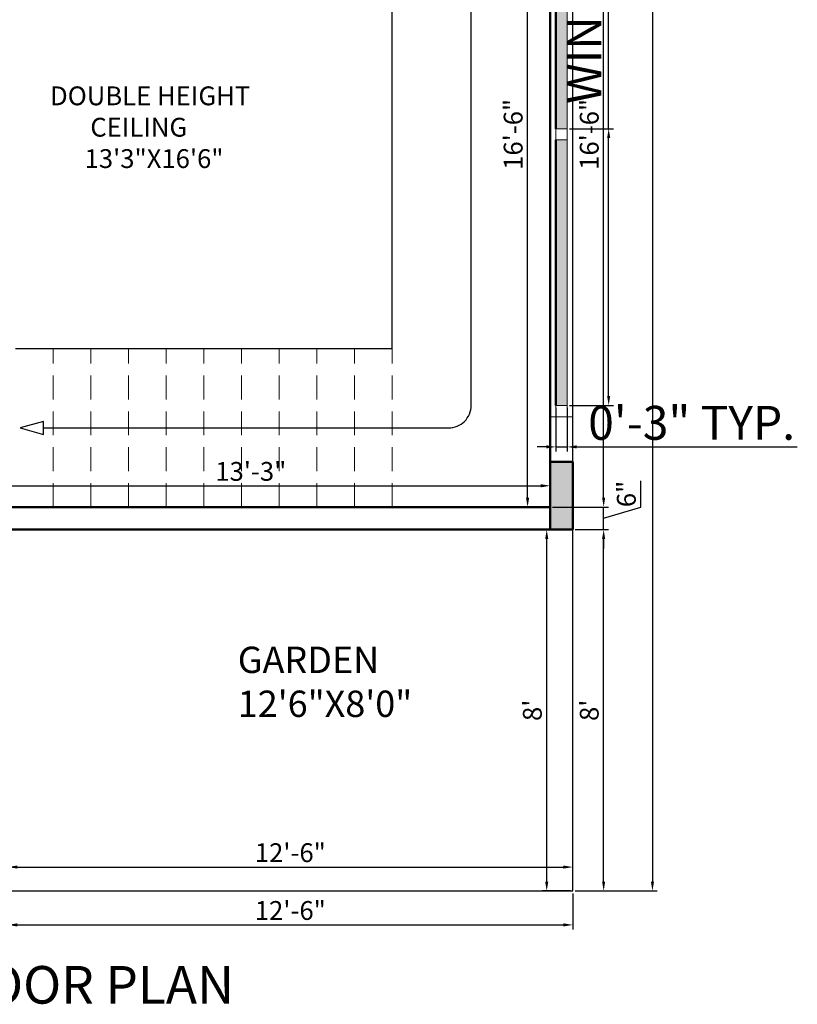
# Model space of a CAD drawing. Units: inches. Extents: x 3064 to 19385, y 846 to 15425.
# Tile 83 of 108: x 7295 to 7501, y 850 to 1112. Entities that reach past the tile are written whole.
import ezdxf

# ---------------------------------------------------------------- set-up
doc = ezdxf.new("R2010")
doc.units = ezdxf.units.IN
doc.linetypes.add('DASHED', pattern=[19.05, 12.7, -6.35])
for name, color, linetype, lineweight in [('A-ANNO-DIMS', 2, 'Continuous', 18), ('A-ANNO-TEXT', 7, 'Continuous', 25), ('A-AREA-IDEN', 3, 'Continuous', 18), ('A-COLS', 1, 'Continuous', 35), ('A-FLOR-STRS', 2, 'Continuous', 25), ('A-FLOR-STRS-OVHD', 2, 'DASHED', 18), ('A-GLAZ', 4, 'Continuous', 18), ('A-WALL', 7, 'Continuous', 50), ('C-PROP', 6, 'Continuous', 25)]:
    doc.layers.add(name, color=color, linetype=linetype, lineweight=lineweight)
doc.styles.get("Standard").update_dxf_attribs({"font": 'arial.ttf'})
doc.dimstyles.new('ISO-25', dxfattribs={"dimtxt": 9, "dimasz": 2.5, "dimexe": 1.25, "dimexo": 0.625, "dimtad": 1, "dimdec": 1, "dimlunit": 3, "dimtxsty": 'Standard', "dimcen": 2.5, "dimadec": 0, "dimazin": 0, "dimtfac": 1, "dimtdec": 1, "dimtmove": 0, "dimatfit": 3, "dimfxl": 1, "dimarcsym": 0})

# ---------------------------------------------------------------- blocks, each defined once
blk = doc.blocks.new('*D305')
at = {"layer": 'A-ANNO-DIMS', "color": 0, "lineweight": -2, "transparency": 16777216}
for p, q in [((7291.71, 879.71), (7291.71, 870.08)), ((7441.71, 879.71), (7441.71, 870.08)), ((7294.21, 871.33), (7439.21, 871.33))]:
    blk.add_line(p, q, dxfattribs=at)
at = {"layer": 'A-ANNO-DIMS', "color": 0, "transparency": 16777216}
for points in [[(7294.21, 871.75), (7294.21, 870.91), (7291.71, 871.33)], [(7439.21, 871.75), (7439.21, 870.91), (7441.71, 871.33)]]:
    blk.add_solid(points, dxfattribs=at)
at = {"layer": 'Defpoints', "color": 0, "transparency": 16777216}
for p in [(7291.71, 880.34), (7441.71, 880.34), (7441.71, 871.33)]:
    blk.add_point(p, dxfattribs=at)
at = {"layer": 'A-ANNO-DIMS', "color": 0, "transparency": 16777216, "insert": (7366.71, 874.51), "char_height": 5, "attachment_point": 5}
blk.add_mtext('12\'-6"', dxfattribs=at)
blk = doc.blocks.new('*D306')
at = {"layer": 'A-ANNO-DIMS', "color": 0, "lineweight": -2, "transparency": 16777216}
for p, q in [((7442.33, 976.34), (7451.15, 976.34)), ((7449.9, 882.84), (7449.9, 973.84)), ((7442.33, 880.34), (7451.15, 880.34))]:
    blk.add_line(p, q, dxfattribs=at)
at = {"layer": 'A-ANNO-DIMS', "color": 0, "transparency": 16777216}
for points in [[(7449.48, 973.84), (7450.31, 973.84), (7449.9, 976.34)], [(7449.48, 882.84), (7450.31, 882.84), (7449.9, 880.34)]]:
    blk.add_solid(points, dxfattribs=at)
at = {"layer": 'Defpoints', "color": 0, "transparency": 16777216}
for p in [(7441.71, 976.34), (7449.9, 976.34), (7441.71, 880.34)]:
    blk.add_point(p, dxfattribs=at)
at = {"layer": 'A-ANNO-DIMS', "color": 0, "transparency": 16777216, "insert": (7446.72, 928.34), "char_height": 5, "attachment_point": 5, "rotation": 90}
blk.add_mtext("8'", dxfattribs=at)
blk = doc.blocks.new('*D307')
at = {"layer": 'A-ANNO-DIMS', "color": 0, "lineweight": -2, "transparency": 16777216}
for p, q in [((7459.74, 982.29), (7459.74, 989.32)), ((7449.9, 984.84), (7449.9, 987.34)), ((7436.33, 982.34), (7451.15, 982.34)), ((7449.9, 976.34), (7449.9, 982.34)), ((7449.9, 976.34), (7449.9, 982.34)), ((7449.9, 979.34), (7459.74, 982.29)), ((7442.33, 976.34), (7451.15, 976.34)), ((7449.9, 973.84), (7449.9, 971.34))]:
    blk.add_line(p, q, dxfattribs=at)
at = {"layer": 'A-ANNO-DIMS', "color": 0, "transparency": 16777216}
for points in [[(7449.48, 984.84), (7450.31, 984.84), (7449.9, 982.34)], [(7449.48, 973.84), (7450.31, 973.84), (7449.9, 976.34)]]:
    blk.add_solid(points, dxfattribs=at)
at = {"layer": 'Defpoints', "color": 0, "transparency": 16777216}
for p in [(7435.71, 982.34), (7449.9, 982.34), (7441.71, 976.34)]:
    blk.add_point(p, dxfattribs=at)
at = {"layer": 'A-ANNO-DIMS', "color": 0, "transparency": 16777216, "insert": (7456.57, 985.81), "char_height": 5, "attachment_point": 5, "rotation": 90}
blk.add_mtext('6"', dxfattribs=at)
blk = doc.blocks.new('*D308')
at = {"layer": 'A-ANNO-DIMS', "color": 0, "lineweight": -2, "transparency": 16777216}
for p, q in [((7436.33, 1180.34), (7451.15, 1180.34)), ((7449.9, 984.84), (7449.9, 1177.84)), ((7436.33, 982.34), (7451.15, 982.34))]:
    blk.add_line(p, q, dxfattribs=at)
at = {"layer": 'A-ANNO-DIMS', "color": 0, "transparency": 16777216}
for points in [[(7449.48, 1177.84), (7450.31, 1177.84), (7449.9, 1180.34)], [(7449.48, 984.84), (7450.31, 984.84), (7449.9, 982.34)]]:
    blk.add_solid(points, dxfattribs=at)
at = {"layer": 'Defpoints', "color": 0, "transparency": 16777216}
for p in [(7435.71, 1180.34), (7449.9, 1180.34), (7435.71, 982.34)]:
    blk.add_point(p, dxfattribs=at)
at = {"layer": 'A-ANNO-DIMS', "color": 0, "transparency": 16777216, "insert": (7446.72, 1081.34), "char_height": 5, "attachment_point": 5, "rotation": 90}
blk.add_mtext('16\'-6"', dxfattribs=at)
blk = doc.blocks.new('*D314')
at = {"layer": 'A-ANNO-DIMS', "color": 0, "lineweight": -2, "transparency": 16777216}
for p, q in [((7442.33, 1396.34), (7464.1, 1396.34)), ((7462.85, 1393.84), (7462.85, 882.84)), ((7442.33, 880.34), (7464.1, 880.34))]:
    blk.add_line(p, q, dxfattribs=at)
at = {"layer": 'A-ANNO-DIMS', "color": 0, "transparency": 16777216}
for points in [[(7462.43, 1393.84), (7463.27, 1393.84), (7462.85, 1396.34)], [(7462.43, 882.84), (7463.27, 882.84), (7462.85, 880.34)]]:
    blk.add_solid(points, dxfattribs=at)
at = {"layer": 'Defpoints', "color": 0, "transparency": 16777216}
for p in [(7441.71, 1396.34), (7441.71, 880.34), (7462.85, 880.34)]:
    blk.add_point(p, dxfattribs=at)
at = {"layer": 'A-ANNO-DIMS', "color": 0, "transparency": 16777216, "insert": (7459.67, 1138.34), "char_height": 5, "attachment_point": 5, "rotation": 90}
blk.add_mtext("43'", dxfattribs=at)
blk = doc.blocks.new('*D274')
at = {"layer": 'A-ANNO-DIMS', "color": 0, "lineweight": -2, "transparency": 16777216}
for p, q in [((7276.71, 982.96), (7276.71, 989.23)), ((7435.71, 982.96), (7435.71, 989.23)), ((7279.21, 987.98), (7433.21, 987.98))]:
    blk.add_line(p, q, dxfattribs=at)
at = {"layer": 'A-ANNO-DIMS', "color": 0, "transparency": 16777216}
for points in [[(7279.21, 988.4), (7279.21, 987.57), (7276.71, 987.98)], [(7433.21, 988.4), (7433.21, 987.57), (7435.71, 987.98)]]:
    blk.add_solid(points, dxfattribs=at)
at = {"layer": 'Defpoints', "color": 0, "transparency": 16777216}
for p in [(7435.71, 987.98), (7276.71, 982.34), (7435.71, 982.34)]:
    blk.add_point(p, dxfattribs=at)
at = {"layer": 'A-ANNO-DIMS', "color": 0, "transparency": 16777216, "insert": (7356.21, 991.16), "char_height": 5, "attachment_point": 5}
blk.add_mtext('13\'-3"', dxfattribs=at)
blk = doc.blocks.new('*D237')
at = {"layer": 'A-ANNO-DIMS', "color": 0, "lineweight": -2, "transparency": 16777216}
for p, q in [((7435.08, 1180.34), (7428.45, 1180.34)), ((7429.7, 984.84), (7429.7, 1177.84)), ((7435.08, 982.34), (7428.45, 982.34))]:
    blk.add_line(p, q, dxfattribs=at)
at = {"layer": 'A-ANNO-DIMS', "color": 0, "transparency": 16777216}
for points in [[(7429.28, 1177.84), (7430.12, 1177.84), (7429.7, 1180.34)], [(7429.28, 984.84), (7430.12, 984.84), (7429.7, 982.34)]]:
    blk.add_solid(points, dxfattribs=at)
at = {"layer": 'Defpoints', "color": 0, "transparency": 16777216}
for p in [(7429.7, 1180.34), (7435.71, 1180.34), (7435.71, 982.34)]:
    blk.add_point(p, dxfattribs=at)
at = {"layer": 'A-ANNO-DIMS', "color": 0, "transparency": 16777216, "insert": (7426.52, 1081.34), "char_height": 5, "attachment_point": 5, "rotation": 90}
blk.add_mtext('16\'-6"', dxfattribs=at)
blk = doc.blocks.new('*D221')
at = {"layer": 'A-ANNO-DIMS', "color": 0, "lineweight": -2, "transparency": 16777216}
for p, q in [((7291.71, 880.96), (7291.71, 887.94)), ((7441.71, 880.96), (7441.71, 887.94)), ((7294.21, 886.69), (7439.21, 886.69))]:
    blk.add_line(p, q, dxfattribs=at)
at = {"layer": 'A-ANNO-DIMS', "color": 0, "transparency": 16777216}
for points in [[(7294.21, 887.11), (7294.21, 886.28), (7291.71, 886.69)], [(7439.21, 887.11), (7439.21, 886.28), (7441.71, 886.69)]]:
    blk.add_solid(points, dxfattribs=at)
at = {"layer": 'Defpoints', "color": 0, "transparency": 16777216}
for p in [(7441.71, 886.69), (7291.71, 880.34), (7441.71, 880.34)]:
    blk.add_point(p, dxfattribs=at)
at = {"layer": 'A-ANNO-DIMS', "color": 0, "transparency": 16777216, "insert": (7366.71, 889.87), "char_height": 5, "attachment_point": 5}
blk.add_mtext('12\'-6"', dxfattribs=at)
blk = doc.blocks.new('*D264')
at = {"layer": 'A-ANNO-DIMS', "color": 0, "lineweight": -2, "transparency": 16777216}
for p, q in [((7441.08, 976.34), (7433.53, 976.34)), ((7434.78, 882.84), (7434.78, 973.84)), ((7441.08, 880.34), (7433.53, 880.34))]:
    blk.add_line(p, q, dxfattribs=at)
at = {"layer": 'A-ANNO-DIMS', "color": 0, "transparency": 16777216}
for points in [[(7434.37, 973.84), (7435.2, 973.84), (7434.78, 976.34)], [(7434.37, 882.84), (7435.2, 882.84), (7434.78, 880.34)]]:
    blk.add_solid(points, dxfattribs=at)
at = {"layer": 'Defpoints', "color": 0, "transparency": 16777216}
for p in [(7434.78, 976.34), (7441.71, 976.34), (7441.71, 880.34)]:
    blk.add_point(p, dxfattribs=at)
at = {"layer": 'A-ANNO-DIMS', "color": 0, "transparency": 16777216, "insert": (7431.61, 928.34), "char_height": 5, "attachment_point": 5, "rotation": 90}
blk.add_mtext("8'", dxfattribs=at)
blk = doc.blocks.new('WIN-1800-PAIR')
h = blk.add_hatch(color=256)
h.dxf.hatch_style = 1
h.paths.add_polyline_path([(0, 0), (3, 0), (3, 70.5), (0, 70.5)])
h.paths.add_polyline_path([(3, 144), (0, 144), (0, 73.5), (3, 73.5)])
blk.add_line((3, 144), (3, 73.5))
blk.add_lwpolyline([(3, 144), (0, 144), (0, 147), (3, 147)], close=True)
blk = doc.blocks.new('WIN-2000')
blk.add_line((3, 0), (3, 70.5))
blk.add_lwpolyline([(3, 70.5), (0, 70.5), (0, 73.5), (3, 73.5)], close=True)
blk = doc.blocks.new('*D447')
at = {"layer": 'A-ANNO-DIMS', "color": 0, "lineweight": -2, "transparency": 16777216}
for p, q in [((7451.23, 1082.84), (7451.23, 1264.78)), ((7440.83, 1082.84), (7452.48, 1082.84)), ((7451.23, 1011.84), (7451.23, 1080.34)), ((7440.83, 1009.34), (7452.48, 1009.34))]:
    blk.add_line(p, q, dxfattribs=at)
at = {"layer": 'A-ANNO-DIMS', "color": 0, "transparency": 16777216}
for points in [[(7450.81, 1080.34), (7451.65, 1080.34), (7451.23, 1082.84)], [(7450.81, 1011.84), (7451.65, 1011.84), (7451.23, 1009.34)]]:
    blk.add_solid(points, dxfattribs=at)
at = {"layer": 'Defpoints', "color": 0, "transparency": 16777216}
for p in [(7440.21, 1082.84), (7451.23, 1082.84), (7440.21, 1009.34)]:
    blk.add_point(p, dxfattribs=at)
at = {"layer": 'A-ANNO-DIMS', "color": 0, "transparency": 16777216, "insert": (7445.95, 1175.06), "char_height": 9, "attachment_point": 5, "rotation": 90}
blk.add_mtext('WINDOW W2000 6\'-1 1/2" TYP.', dxfattribs=at)
blk = doc.blocks.new('*D448')
at = {"layer": 'A-ANNO-DIMS', "color": 0, "lineweight": -2, "transparency": 16777216}
for p, q in [((7437.21, 1008.71), (7437.21, 997.06)), ((7440.21, 1008.71), (7440.21, 997.06)), ((7434.71, 998.31), (7432.21, 998.31)), ((7437.21, 998.31), (7440.21, 998.31)), ((7442.71, 998.31), (7501.31, 998.31))]:
    blk.add_line(p, q, dxfattribs=at)
at = {"layer": 'A-ANNO-DIMS', "color": 0, "transparency": 16777216}
for points in [[(7434.71, 998.73), (7434.71, 997.9), (7437.21, 998.31)], [(7442.71, 998.73), (7442.71, 997.9), (7440.21, 998.31)]]:
    blk.add_solid(points, dxfattribs=at)
at = {"layer": 'Defpoints', "color": 0, "transparency": 16777216}
for p in [(7437.21, 1009.34), (7440.21, 1009.34), (7440.21, 998.31)]:
    blk.add_point(p, dxfattribs=at)
at = {"layer": 'A-ANNO-DIMS', "color": 0, "transparency": 16777216, "insert": (7473.26, 1003.54), "char_height": 9, "attachment_point": 5}
blk.add_mtext('0\'-3" TYP.', dxfattribs=at)

msp = doc.modelspace()

# ---------------------------------------------------------------- hatches: boundary and pattern name
at = {"layer": 'A-COLS'}
h = msp.add_hatch(color=256, dxfattribs=at)
h.dxf.hatch_style = 1
h.paths.add_polyline_path([(7435.71, 976.34), (7441.71, 976.34), (7441.71, 994.34), (7435.71, 994.34)])

# ---------------------------------------------------------------- linework, layer by layer
at = {"layer": 'A-FLOR-STRS'}
for q in [(7393.71, 1180.34), (7293.71, 1024.34)]:
    msp.add_line((7393.71, 1024.34), q, dxfattribs=at)
msp.add_lwpolyline([(7301.19, 1003.34), (7408.71, 1003.34, 0.414214), (7414.71, 1009.34), (7414.71, 1153.34, 0.414214), (7408.71, 1159.34), (7281.71, 1159.34)], format="xyb", dxfattribs=at)
msp.add_lwpolyline([(7295, 1003.34), (7301.19, 1001.61), (7301.19, 1005.07)], close=True, dxfattribs=at)
at = {"layer": 'A-FLOR-STRS-OVHD', "ltscale": 0.5}
for p, q in [((7303.71, 982.34), (7303.71, 1024.34)), ((7313.71, 982.34), (7313.71, 1024.34)), ((7323.71, 982.34), (7323.71, 1024.34)), ((7333.71, 982.34), (7333.71, 1024.34)), ((7343.71, 982.34), (7343.71, 1024.34)), ((7353.71, 982.34), (7353.71, 1024.34)), ((7363.71, 982.34), (7363.71, 1024.34)), ((7373.71, 982.34), (7373.71, 1024.34)), ((7383.71, 982.34), (7383.71, 1024.34)), ((7393.71, 982.34), (7393.71, 1024.34))]:
    msp.add_line(p, q, dxfattribs=at)
at = {"layer": 'A-GLAZ'}
msp.add_line((7441.71, 1006.34), (7435.71, 1006.34), dxfattribs=at)
msp.add_line((7441.71, 1006.34), (7435.71, 1006.34), dxfattribs=at)
msp.add_lwpolyline([(7440.21, 1006.34), (7437.21, 1006.34), (7437.21, 1009.34), (7440.21, 1009.34)], close=True, dxfattribs=at)
at = {"layer": 'A-WALL'}
for p, q in [((7435.71, 982.34), (7435.71, 1180.34)), ((7437.21, 1153.34), (7437.21, 1082.84)), ((7437.21, 1009.34), (7437.21, 1079.84)), ((7435.71, 982.34), (7276.71, 982.34)), ((7441.71, 976.34), (7276.71, 976.34))]:
    msp.add_line(p, q, dxfattribs=at)
msp.add_lwpolyline([(7441.71, 976.34), (7441.71, 994.34), (7435.71, 994.34), (7435.71, 976.34)], close=True, dxfattribs=at)
at = {"layer": 'C-PROP'}
for p, q in [((7441.71, 880.34), (7441.71, 1396.34)), ((7099.71, 880.34), (7441.71, 880.34))]:
    msp.add_line(p, q, dxfattribs=at)

# ---------------------------------------------------------------- block references
at = {"layer": 'A-GLAZ'}
for name in ['WIN-1800-PAIR', 'WIN-2000']:
    msp.add_blockref(name, (7437.2, 1009.34), dxfattribs=at)

# ---------------------------------------------------------------- texts
at = {"layer": 'A-ANNO-TEXT', "insert": (7210.37, 860.41), "char_height": 10, "attachment_point": 1}
msp.add_mtext_dynamic_manual_height_columns('GROUND FLOOR PLAN', width=200.9739, gutter_width=12.5, heights=[0], dxfattribs=at)
at = {"layer": 'A-AREA-IDEN', "attachment_point": 1}
for s, width, insert, char_height in [('DOUBLE HEIGHT \\P       CEILING            \\P      13\'3"X16\'6"', 57.0817, (7302.91, 1094.07), 5), ('GARDEN\\P12\'6"X8\'0"', 67.5924, (7352.75, 945.24), 7)]:
    msp.add_mtext_dynamic_manual_height_columns(s, width=width, gutter_width=12.5, heights=[0], dxfattribs=dict(at, insert=insert, char_height=char_height))

# ---------------------------------------------------------------- dimensions: what is measured, and where the dimension line sits
at = {"layer": 'A-ANNO-DIMS'}
for base, p1, p2, override, picture, middle in [((7462.85, 880.34), (7441.71, 1396.34), (7441.71, 880.34), {"dimtxt": 5, "dimclrd": 0, "dimclre": 0, "dimclrt": 0}, '*D314', (7459.67, 1138.34)), ((7429.7, 1180.34), (7435.71, 982.34), (7435.71, 1180.34), {"dimtxt": 5, "dimclrd": 0, "dimclre": 0, "dimclrt": 0}, '*D237', (7426.52, 1081.34)), ((7449.9, 1180.34), (7435.71, 982.34), (7435.71, 1180.34), {"dimtxt": 5, "dimclrd": 0, "dimclre": 0, "dimclrt": 0, "dimtmove": 1}, '*D308', (7446.72, 1081.34)), ((7449.9, 982.34), (7441.71, 976.34), (7435.71, 982.34), {"dimtxt": 5, "dimclrd": 0, "dimclre": 0, "dimclrt": 0, "dimtmove": 1}, '*D307', (7456.57, 982.92)), ((7434.78, 976.34), (7441.71, 880.34), (7441.71, 976.34), {"dimtxt": 5, "dimclrd": 0, "dimclre": 0, "dimclrt": 0}, '*D264', (7431.61, 928.34)), ((7449.9, 976.34), (7441.71, 880.34), (7441.71, 976.34), {"dimtxt": 5, "dimclrd": 0, "dimclre": 0, "dimclrt": 0}, '*D306', (7446.72, 928.34))]:
    dim = msp.add_linear_dim(base=base, p1=p1, p2=p2, angle=90, dimstyle='ISO-25', override=override, dxfattribs=at)
    dim.commit()
    dim.dimension.update_dxf_attribs({"geometry": picture, "text_midpoint": middle})
dim = msp.add_linear_dim(base=(7451.23, 1082.84), p1=(7440.21, 1009.34), p2=(7440.21, 1082.84), angle=90, text='WINDOW W2000 <> TYP.', dimstyle='ISO-25', override={"dimdec": 1, "dimrnd": 0, "dimzin": 1, "dimlunit": 4, "dimfrac": 2}, dxfattribs=at)
dim.commit()
dim.dimension.update_dxf_attribs({"geometry": '*D447', "text_midpoint": (7445.95, 1175.06)})
dim = msp.add_linear_dim(base=(7440.21, 998.31), p1=(7437.21, 1009.34), p2=(7440.21, 1009.34), text='<> TYP.', dimstyle='ISO-25', override={"dimdec": 1, "dimrnd": 0, "dimzin": 1, "dimlunit": 4, "dimfrac": 2}, dxfattribs=at)
dim.commit()
dim.dimension.update_dxf_attribs({"geometry": '*D448', "text_midpoint": (7473.26, 1003.54)})
for base, p1, p2, override, picture, middle in [((7435.71, 987.98), (7276.71, 982.34), (7435.71, 982.34), {"dimtxt": 5, "dimclrd": 0, "dimclre": 0, "dimclrt": 0, "dimtmove": 1}, '*D274', (7356.21, 991.16)), ((7441.71, 886.69), (7291.71, 880.34), (7441.71, 880.34), {"dimtxt": 5, "dimclrd": 0, "dimclre": 0, "dimclrt": 0}, '*D221', (7366.71, 889.87)), ((7441.71, 871.33), (7291.71, 880.34), (7441.71, 880.34), {"dimtxt": 5, "dimclrd": 0, "dimclre": 0, "dimclrt": 0, "dimtmove": 1}, '*D305', (7366.71, 874.51))]:
    dim = msp.add_linear_dim(base=base, p1=p1, p2=p2, dimstyle='ISO-25', override=override, dxfattribs=at)
    dim.commit()
    dim.dimension.update_dxf_attribs({"geometry": picture, "text_midpoint": middle})

doc.saveas('drawing.dxf')
